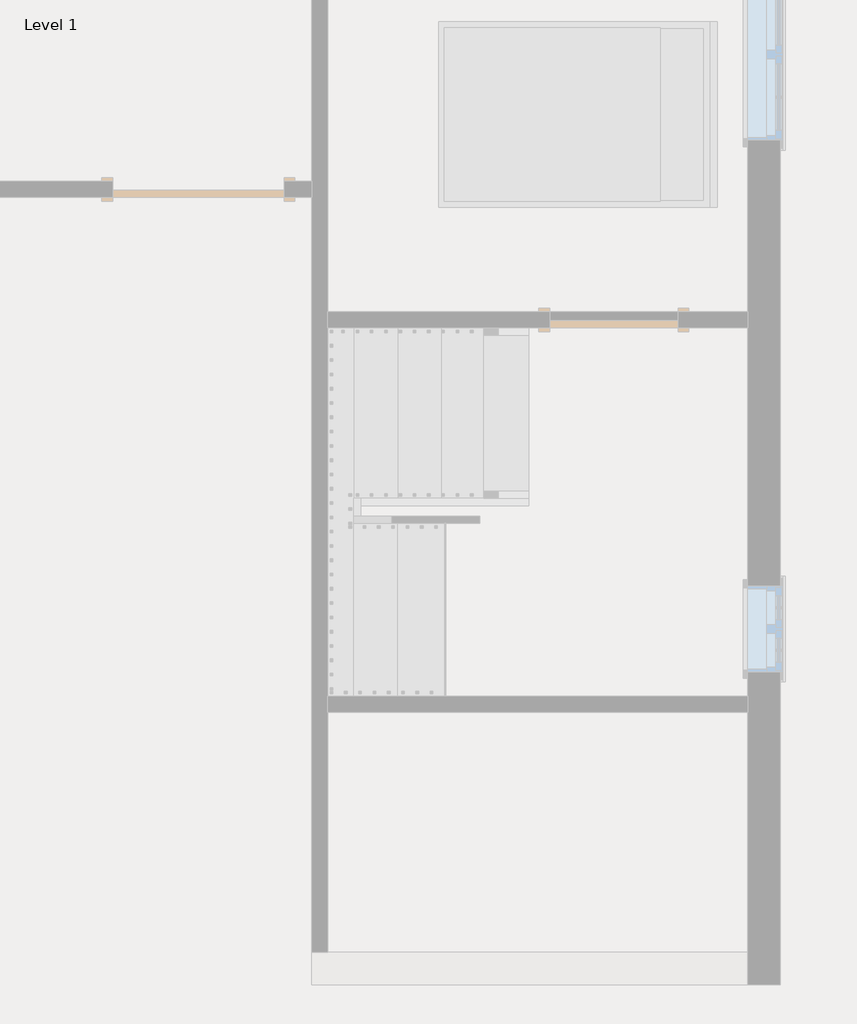
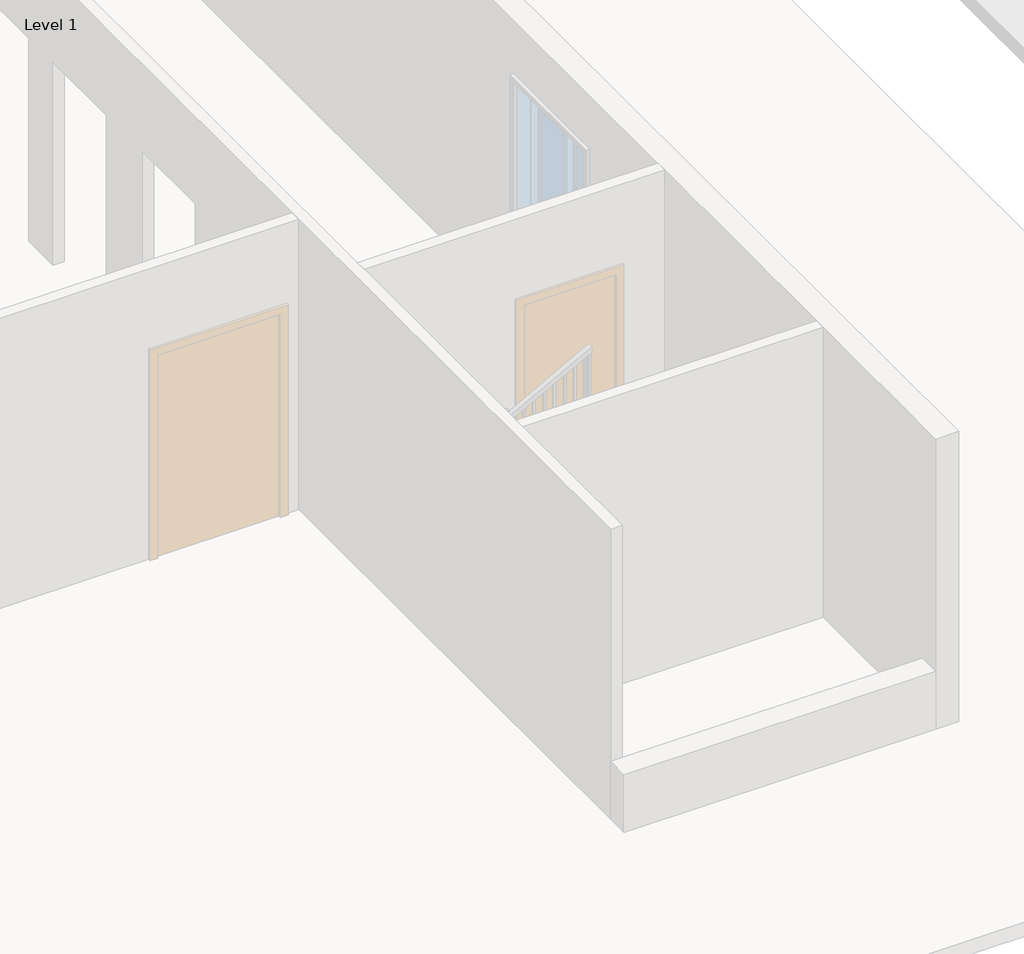
# One storey, part 4 of 7: 2 railings.
"""IFC4 building model written with IfcOpenShell, lengths in millimetres."""

from ifc_helpers import new_model, si_unit, frame, origin, place, context, project, spatial, polyline, outline, extrude, faceted_brep, element, save

model = new_model("IFC4")

# Units and contexts
model_context = context("Model", 3, world=origin())
ifc_project = project(units=[si_unit("LENGTHUNIT", "METRE", prefix="MILLI")], contexts=[model_context])

# Site, building, storey
site = spatial("IfcSite", under=ifc_project)
building = spatial("IfcBuilding", under=site)
storey = spatial("IfcBuildingStorey", under=building, Name="Level 1", Elevation=0.0)

# Railings
placement = place(None, origin())
element("IfcRailing", 1, ObjectType="Handrail - Rectangular", at=placement, inside=storey, context=model_context, shape_type="SolidModel", body=[
    faceted_brep([(7105.1820958, 5435.6, 1083.7333333), (7105.1820958, 5435.6, 1025.8977421), (7105.1820958, 5486.4, 1025.8977421), (7105.1820958, 5486.4, 1083.7333333), (5860.5820958, 5435.6, 1761.0666667), (5847.654197, 5435.6, 1710.2666667), (5847.654197, 5486.4, 1710.2666667), (5860.5820958, 5486.4, 1761.0666667), (5727.7, 5435.6, 1761.0666667), (5727.7, 5435.6, 1710.2666667), (5676.9, 5486.4, 1710.2666667), (5676.9, 5486.4, 1761.0666667), (5727.7, 2997.2, 1761.0666667), (5727.7, 2946.4, 1710.2666667), (5676.9, 2946.4, 1710.2666667), (5676.9, 2997.2, 1761.0666667), (5727.7, 2997.2, 1899.5526009), (5727.7, 2946.4, 1848.7526009), (5676.9, 2946.4, 1848.7526009), (5676.9, 2997.2, 1899.5526009), (5727.7, 2921.0, 1899.5526009), (5727.7, 2921.0, 1848.7526009), (5676.9, 2870.2, 1848.7526009), (5676.9, 2870.2, 1899.5526009), (5803.9, 2921.0, 1899.5526009), (5816.8278988, 2921.0, 1848.7526009), (5816.8278988, 2870.2, 1848.7526009), (5803.9, 2870.2, 1899.5526009), (7105.1820958, 2921.0, 2607.7333333), (7105.1820958, 2870.2, 2607.7333333), (7105.1820958, 2870.2, 2549.8977421), (7105.1820958, 2921.0, 2549.8977421)], [[[0, 1, 2, 3]], [[1, 0, 4, 5]], [[2, 1, 5, 6]], [[3, 2, 6, 7]], [[0, 3, 7, 4]], [[5, 4, 8, 9]], [[6, 5, 9, 10]], [[7, 6, 10, 11]], [[4, 7, 11, 8]], [[9, 8, 12, 13]], [[10, 9, 13, 14]], [[11, 10, 14, 15]], [[8, 11, 15, 12]], [[13, 12, 16, 17]], [[14, 13, 17, 18]], [[15, 14, 18, 19]], [[12, 15, 19, 16]], [[17, 16, 20, 21]], [[18, 17, 21, 22]], [[19, 18, 22, 23]], [[16, 19, 23, 20]], [[21, 20, 24, 25]], [[22, 21, 25, 26]], [[23, 22, 26, 27]], [[20, 23, 27, 24]], [[28, 29, 30, 31]], [[25, 24, 28, 31]], [[26, 25, 31, 30]], [[27, 26, 30, 29]], [[24, 27, 29, 28]]]),
    extrude(outline(polyline([(2510.4108873, 7032.625), (2500.0435403, 7013.575), (1524.0, 7013.575), (1524.0, 7032.625), (2510.4108873, 7032.625)])), frame((0.0, 2886.075, 0.0), z_axis=(0.0, 1.0, 0.0), x_axis=(0.0, 0.0, 1.0)), (0.0, 0.0, 1.0), 19.05),
    extrude(outline(polyline([(2455.1183703, 6931.025), (2444.7510233, 6911.975), (1524.0, 6911.975), (1524.0, 6931.025), (2455.1183703, 6931.025)])), frame((0.0, 2886.075, 0.0), z_axis=(0.0, 1.0, 0.0), x_axis=(0.0, 0.0, 1.0)), (0.0, 0.0, 1.0), 19.05),
    extrude(outline(polyline([(2399.8258533, 6829.425), (2389.4585063, 6810.375), (1524.0, 6810.375), (1524.0, 6829.425), (2399.8258533, 6829.425)])), frame((0.0, 2886.075, 0.0), z_axis=(0.0, 1.0, 0.0), x_axis=(0.0, 0.0, 1.0)), (0.0, 0.0, 1.0), 19.05),
    extrude(outline(polyline([(2344.5333363, 6727.825), (2334.1659893, 6708.775), (1354.6666667, 6708.775), (1354.6666667, 6727.825), (2344.5333363, 6727.825)])), frame((0.0, 2886.075, 0.0), z_axis=(0.0, 1.0, 0.0), x_axis=(0.0, 0.0, 1.0)), (0.0, 0.0, 1.0), 19.05),
    extrude(outline(polyline([(2289.2408192, 6626.225), (2278.8734723, 6607.175), (1354.6666667, 6607.175), (1354.6666667, 6626.225), (2289.2408192, 6626.225)])), frame((0.0, 2886.075, 0.0), z_axis=(0.0, 1.0, 0.0), x_axis=(0.0, 0.0, 1.0)), (0.0, 0.0, 1.0), 19.05),
    extrude(outline(polyline([(2233.9483022, 6524.625), (2223.5809553, 6505.575), (1354.6666667, 6505.575), (1354.6666667, 6524.625), (2233.9483022, 6524.625)])), frame((0.0, 2886.075, 0.0), z_axis=(0.0, 1.0, 0.0), x_axis=(0.0, 0.0, 1.0)), (0.0, 0.0, 1.0), 19.05),
    extrude(outline(polyline([(2178.6557852, 6423.025), (2168.2884383, 6403.975), (1185.3333333, 6403.975), (1185.3333333, 6423.025), (2178.6557852, 6423.025)])), frame((0.0, 2886.075, 0.0), z_axis=(0.0, 1.0, 0.0), x_axis=(0.0, 0.0, 1.0)), (0.0, 0.0, 1.0), 19.05),
    extrude(outline(polyline([(2123.3632682, 6321.425), (2112.9959213, 6302.375), (1185.3333333, 6302.375), (1185.3333333, 6321.425), (2123.3632682, 6321.425)])), frame((0.0, 2886.075, 0.0), z_axis=(0.0, 1.0, 0.0), x_axis=(0.0, 0.0, 1.0)), (0.0, 0.0, 1.0), 19.05),
    extrude(outline(polyline([(2068.0707512, 6219.825), (2057.7034043, 6200.775), (1185.3333333, 6200.775), (1185.3333333, 6219.825), (2068.0707512, 6219.825)])), frame((0.0, 2886.075, 0.0), z_axis=(0.0, 1.0, 0.0), x_axis=(0.0, 0.0, 1.0)), (0.0, 0.0, 1.0), 19.05),
    extrude(outline(polyline([(2012.7782342, 6118.225), (2002.4108873, 6099.175), (1016.0, 6099.175), (1016.0, 6118.225), (2012.7782342, 6118.225)])), frame((0.0, 2886.075, 0.0), z_axis=(0.0, 1.0, 0.0), x_axis=(0.0, 0.0, 1.0)), (0.0, 0.0, 1.0), 19.05),
    extrude(outline(polyline([(1957.4857172, 6016.625), (1947.1183703, 5997.575), (1016.0, 5997.575), (1016.0, 6016.625), (1957.4857172, 6016.625)])), frame((0.0, 2886.075, 0.0), z_axis=(0.0, 1.0, 0.0), x_axis=(0.0, 0.0, 1.0)), (0.0, 0.0, 1.0), 19.05),
    extrude(outline(polyline([(1902.1932002, 5915.025), (1891.8258533, 5895.975), (1016.0, 5895.975), (1016.0, 5915.025), (1902.1932002, 5915.025)])), frame((0.0, 2886.075, 0.0), z_axis=(0.0, 1.0, 0.0), x_axis=(0.0, 0.0, 1.0)), (0.0, 0.0, 1.0), 19.05),
    extrude(outline(polyline([(1846.9006832, 5813.425), (1836.5333363, 5794.375), (846.6666667, 5794.375), (846.6666667, 5813.425), (1846.9006832, 5813.425)])), frame((0.0, 2886.075, 0.0), z_axis=(0.0, 1.0, 0.0), x_axis=(0.0, 0.0, 1.0)), (0.0, 0.0, 1.0), 19.05),
    extrude(outline(polyline([(5692.775, 2930.525), (5711.825, 2930.525), (5711.825, 2911.475), (5692.775, 2911.475), (5692.775, 2930.525)])), frame((0.0, 0.0, 846.6666667), z_axis=(0.0, 0.0, 1.0), x_axis=(1.0, 0.0, 0.0)), (0.0, 0.0, 1.0), 1002.0859343),
    extrude(outline(polyline([(5692.775, 3032.125), (5711.825, 3032.125), (5711.825, 3013.075), (5692.775, 3013.075), (5692.775, 3032.125)])), frame((0.0, 0.0, 846.6666667), z_axis=(0.0, 0.0, 1.0), x_axis=(1.0, 0.0, 0.0)), (0.0, 0.0, 1.0), 863.6),
    extrude(outline(polyline([(5692.775, 3133.725), (5711.825, 3133.725), (5711.825, 3114.675), (5692.775, 3114.675), (5692.775, 3133.725)])), frame((0.0, 0.0, 846.6666667), z_axis=(0.0, 0.0, 1.0), x_axis=(1.0, 0.0, 0.0)), (0.0, 0.0, 1.0), 863.6),
    extrude(outline(polyline([(5692.775, 3235.325), (5711.825, 3235.325), (5711.825, 3216.275), (5692.775, 3216.275), (5692.775, 3235.325)])), frame((0.0, 0.0, 846.6666667), z_axis=(0.0, 0.0, 1.0), x_axis=(1.0, 0.0, 0.0)), (0.0, 0.0, 1.0), 863.6),
    extrude(outline(polyline([(5692.775, 3336.925), (5711.825, 3336.925), (5711.825, 3317.875), (5692.775, 3317.875), (5692.775, 3336.925)])), frame((0.0, 0.0, 846.6666667), z_axis=(0.0, 0.0, 1.0), x_axis=(1.0, 0.0, 0.0)), (0.0, 0.0, 1.0), 863.6),
    extrude(outline(polyline([(5692.775, 3438.525), (5711.825, 3438.525), (5711.825, 3419.475), (5692.775, 3419.475), (5692.775, 3438.525)])), frame((0.0, 0.0, 846.6666667), z_axis=(0.0, 0.0, 1.0), x_axis=(1.0, 0.0, 0.0)), (0.0, 0.0, 1.0), 863.6),
    extrude(outline(polyline([(5692.775, 3540.125), (5711.825, 3540.125), (5711.825, 3521.075), (5692.775, 3521.075), (5692.775, 3540.125)])), frame((0.0, 0.0, 846.6666667), z_axis=(0.0, 0.0, 1.0), x_axis=(1.0, 0.0, 0.0)), (0.0, 0.0, 1.0), 863.6),
    extrude(outline(polyline([(5692.775, 3641.725), (5711.825, 3641.725), (5711.825, 3622.675), (5692.775, 3622.675), (5692.775, 3641.725)])), frame((0.0, 0.0, 846.6666667), z_axis=(0.0, 0.0, 1.0), x_axis=(1.0, 0.0, 0.0)), (0.0, 0.0, 1.0), 863.6),
    extrude(outline(polyline([(5692.775, 3743.325), (5711.825, 3743.325), (5711.825, 3724.275), (5692.775, 3724.275), (5692.775, 3743.325)])), frame((0.0, 0.0, 846.6666667), z_axis=(0.0, 0.0, 1.0), x_axis=(1.0, 0.0, 0.0)), (0.0, 0.0, 1.0), 863.6),
    extrude(outline(polyline([(5692.775, 3844.925), (5711.825, 3844.925), (5711.825, 3825.875), (5692.775, 3825.875), (5692.775, 3844.925)])), frame((0.0, 0.0, 846.6666667), z_axis=(0.0, 0.0, 1.0), x_axis=(1.0, 0.0, 0.0)), (0.0, 0.0, 1.0), 863.6),
    extrude(outline(polyline([(5692.775, 3946.525), (5711.825, 3946.525), (5711.825, 3927.475), (5692.775, 3927.475), (5692.775, 3946.525)])), frame((0.0, 0.0, 846.6666667), z_axis=(0.0, 0.0, 1.0), x_axis=(1.0, 0.0, 0.0)), (0.0, 0.0, 1.0), 863.6),
    extrude(outline(polyline([(5692.775, 4048.125), (5711.825, 4048.125), (5711.825, 4029.075), (5692.775, 4029.075), (5692.775, 4048.125)])), frame((0.0, 0.0, 846.6666667), z_axis=(0.0, 0.0, 1.0), x_axis=(1.0, 0.0, 0.0)), (0.0, 0.0, 1.0), 863.6),
    extrude(outline(polyline([(5692.775, 4149.725), (5711.825, 4149.725), (5711.825, 4130.675), (5692.775, 4130.675), (5692.775, 4149.725)])), frame((0.0, 0.0, 846.6666667), z_axis=(0.0, 0.0, 1.0), x_axis=(1.0, 0.0, 0.0)), (0.0, 0.0, 1.0), 863.6),
    extrude(outline(polyline([(5692.775, 4251.325), (5711.825, 4251.325), (5711.825, 4232.275), (5692.775, 4232.275), (5692.775, 4251.325)])), frame((0.0, 0.0, 846.6666667), z_axis=(0.0, 0.0, 1.0), x_axis=(1.0, 0.0, 0.0)), (0.0, 0.0, 1.0), 863.6),
    extrude(outline(polyline([(5692.775, 4352.925), (5711.825, 4352.925), (5711.825, 4333.875), (5692.775, 4333.875), (5692.775, 4352.925)])), frame((0.0, 0.0, 846.6666667), z_axis=(0.0, 0.0, 1.0), x_axis=(1.0, 0.0, 0.0)), (0.0, 0.0, 1.0), 863.6),
    extrude(outline(polyline([(5692.775, 4454.525), (5711.825, 4454.525), (5711.825, 4435.475), (5692.775, 4435.475), (5692.775, 4454.525)])), frame((0.0, 0.0, 846.6666667), z_axis=(0.0, 0.0, 1.0), x_axis=(1.0, 0.0, 0.0)), (0.0, 0.0, 1.0), 863.6),
    extrude(outline(polyline([(5692.775, 4556.125), (5711.825, 4556.125), (5711.825, 4537.075), (5692.775, 4537.075), (5692.775, 4556.125)])), frame((0.0, 0.0, 846.6666667), z_axis=(0.0, 0.0, 1.0), x_axis=(1.0, 0.0, 0.0)), (0.0, 0.0, 1.0), 863.6),
    extrude(outline(polyline([(5692.775, 4657.725), (5711.825, 4657.725), (5711.825, 4638.675), (5692.775, 4638.675), (5692.775, 4657.725)])), frame((0.0, 0.0, 846.6666667), z_axis=(0.0, 0.0, 1.0), x_axis=(1.0, 0.0, 0.0)), (0.0, 0.0, 1.0), 863.6),
    extrude(outline(polyline([(5692.775, 4759.325), (5711.825, 4759.325), (5711.825, 4740.275), (5692.775, 4740.275), (5692.775, 4759.325)])), frame((0.0, 0.0, 846.6666667), z_axis=(0.0, 0.0, 1.0), x_axis=(1.0, 0.0, 0.0)), (0.0, 0.0, 1.0), 863.6),
    extrude(outline(polyline([(5692.775, 4860.925), (5711.825, 4860.925), (5711.825, 4841.875), (5692.775, 4841.875), (5692.775, 4860.925)])), frame((0.0, 0.0, 846.6666667), z_axis=(0.0, 0.0, 1.0), x_axis=(1.0, 0.0, 0.0)), (0.0, 0.0, 1.0), 863.6),
    extrude(outline(polyline([(5692.775, 4962.525), (5711.825, 4962.525), (5711.825, 4943.475), (5692.775, 4943.475), (5692.775, 4962.525)])), frame((0.0, 0.0, 846.6666667), z_axis=(0.0, 0.0, 1.0), x_axis=(1.0, 0.0, 0.0)), (0.0, 0.0, 1.0), 863.6),
    extrude(outline(polyline([(5692.775, 5064.125), (5711.825, 5064.125), (5711.825, 5045.075), (5692.775, 5045.075), (5692.775, 5064.125)])), frame((0.0, 0.0, 846.6666667), z_axis=(0.0, 0.0, 1.0), x_axis=(1.0, 0.0, 0.0)), (0.0, 0.0, 1.0), 863.6),
    extrude(outline(polyline([(5692.775, 5165.725), (5711.825, 5165.725), (5711.825, 5146.675), (5692.775, 5146.675), (5692.775, 5165.725)])), frame((0.0, 0.0, 846.6666667), z_axis=(0.0, 0.0, 1.0), x_axis=(1.0, 0.0, 0.0)), (0.0, 0.0, 1.0), 863.6),
    extrude(outline(polyline([(5692.775, 5267.325), (5711.825, 5267.325), (5711.825, 5248.275), (5692.775, 5248.275), (5692.775, 5267.325)])), frame((0.0, 0.0, 846.6666667), z_axis=(0.0, 0.0, 1.0), x_axis=(1.0, 0.0, 0.0)), (0.0, 0.0, 1.0), 863.6),
    extrude(outline(polyline([(5692.775, 5368.925), (5711.825, 5368.925), (5711.825, 5349.875), (5692.775, 5349.875), (5692.775, 5368.925)])), frame((0.0, 0.0, 846.6666667), z_axis=(0.0, 0.0, 1.0), x_axis=(1.0, 0.0, 0.0)), (0.0, 0.0, 1.0), 863.6),
    extrude(outline(polyline([(5793.9070958, 5470.525), (5793.9070958, 5451.475), (5774.8570958, 5451.475), (5774.8570958, 5470.525), (5793.9070958, 5470.525)])), frame((0.0, 0.0, 846.6666667), z_axis=(0.0, 0.0, 1.0), x_axis=(1.0, 0.0, 0.0)), (0.0, 0.0, 1.0), 863.6),
    extrude(outline(polyline([(1684.2242727, 5895.5070958), (1694.5916197, 5876.4570958), (677.3333333, 5876.4570958), (677.3333333, 5895.5070958), (1684.2242727, 5895.5070958)])), frame((0.0, 5451.475, 0.0), z_axis=(0.0, 1.0, 0.0), x_axis=(0.0, 0.0, 1.0)), (0.0, 0.0, 1.0), 19.05),
    extrude(outline(polyline([(1628.9317557, 5997.1070958), (1639.2991027, 5978.0570958), (677.3333333, 5978.0570958), (677.3333333, 5997.1070958), (1628.9317557, 5997.1070958)])), frame((0.0, 5451.475, 0.0), z_axis=(0.0, 1.0, 0.0), x_axis=(0.0, 0.0, 1.0)), (0.0, 0.0, 1.0), 19.05),
    extrude(outline(polyline([(1573.6392387, 6098.7070958), (1584.0065857, 6079.6570958), (677.3333333, 6079.6570958), (677.3333333, 6098.7070958), (1573.6392387, 6098.7070958)])), frame((0.0, 5451.475, 0.0), z_axis=(0.0, 1.0, 0.0), x_axis=(0.0, 0.0, 1.0)), (0.0, 0.0, 1.0), 19.05),
    extrude(outline(polyline([(1518.3467217, 6200.3070958), (1528.7140687, 6181.2570958), (508.0, 6181.2570958), (508.0, 6200.3070958), (1518.3467217, 6200.3070958)])), frame((0.0, 5451.475, 0.0), z_axis=(0.0, 1.0, 0.0), x_axis=(0.0, 0.0, 1.0)), (0.0, 0.0, 1.0), 19.05),
    extrude(outline(polyline([(1463.0542047, 6301.9070958), (1473.4215517, 6282.8570958), (508.0, 6282.8570958), (508.0, 6301.9070958), (1463.0542047, 6301.9070958)])), frame((0.0, 5451.475, 0.0), z_axis=(0.0, 1.0, 0.0), x_axis=(0.0, 0.0, 1.0)), (0.0, 0.0, 1.0), 19.05),
    extrude(outline(polyline([(1407.7616877, 6403.5070958), (1418.1290347, 6384.4570958), (508.0, 6384.4570958), (508.0, 6403.5070958), (1407.7616877, 6403.5070958)])), frame((0.0, 5451.475, 0.0), z_axis=(0.0, 1.0, 0.0), x_axis=(0.0, 0.0, 1.0)), (0.0, 0.0, 1.0), 19.05),
    extrude(outline(polyline([(1352.4691707, 6505.1070958), (1362.8365176, 6486.0570958), (338.6666667, 6486.0570958), (338.6666667, 6505.1070958), (1352.4691707, 6505.1070958)])), frame((0.0, 5451.475, 0.0), z_axis=(0.0, 1.0, 0.0), x_axis=(0.0, 0.0, 1.0)), (0.0, 0.0, 1.0), 19.05),
    extrude(outline(polyline([(1297.1766537, 6606.7070958), (1307.5440006, 6587.6570958), (338.6666667, 6587.6570958), (338.6666667, 6606.7070958), (1297.1766537, 6606.7070958)])), frame((0.0, 5451.475, 0.0), z_axis=(0.0, 1.0, 0.0), x_axis=(0.0, 0.0, 1.0)), (0.0, 0.0, 1.0), 19.05),
    extrude(outline(polyline([(1241.8841367, 6708.3070958), (1252.2514836, 6689.2570958), (338.6666667, 6689.2570958), (338.6666667, 6708.3070958), (1241.8841367, 6708.3070958)])), frame((0.0, 5451.475, 0.0), z_axis=(0.0, 1.0, 0.0), x_axis=(0.0, 0.0, 1.0)), (0.0, 0.0, 1.0), 19.05),
    extrude(outline(polyline([(1186.5916197, 6809.9070958), (1196.9589666, 6790.8570958), (169.3333333, 6790.8570958), (169.3333333, 6809.9070958), (1186.5916197, 6809.9070958)])), frame((0.0, 5451.475, 0.0), z_axis=(0.0, 1.0, 0.0), x_axis=(0.0, 0.0, 1.0)), (0.0, 0.0, 1.0), 19.05),
    extrude(outline(polyline([(1131.2991027, 6911.5070958), (1141.6664496, 6892.4570958), (169.3333333, 6892.4570958), (169.3333333, 6911.5070958), (1131.2991027, 6911.5070958)])), frame((0.0, 5451.475, 0.0), z_axis=(0.0, 1.0, 0.0), x_axis=(0.0, 0.0, 1.0)), (0.0, 0.0, 1.0), 19.05),
    extrude(outline(polyline([(1076.0065857, 7013.1070958), (1086.3739326, 6994.0570958), (169.3333333, 6994.0570958), (169.3333333, 7013.1070958), (1076.0065857, 7013.1070958)])), frame((0.0, 5451.475, 0.0), z_axis=(0.0, 1.0, 0.0), x_axis=(0.0, 0.0, 1.0)), (0.0, 0.0, 1.0), 19.05),
    extrude(outline(polyline([(5692.775, 2905.125), (5711.825, 2905.125), (5711.825, 2886.075), (5692.775, 2886.075), (5692.775, 2905.125)])), frame((0.0, 0.0, 846.6666667), z_axis=(0.0, 0.0, 1.0), x_axis=(1.0, 0.0, 0.0)), (0.0, 0.0, 1.0), 1002.0859343),
    extrude(outline(polyline([(5711.825, 5470.525), (5711.825, 5451.475), (5692.775, 5451.475), (5692.775, 5470.525), (5711.825, 5470.525)])), frame((0.0, 0.0, 846.6666667), z_axis=(0.0, 0.0, 1.0), x_axis=(1.0, 0.0, 0.0)), (0.0, 0.0, 1.0), 863.6),
    extrude(outline(polyline([(2549.8977421, 7105.1820958), (2539.5303952, 7086.1320958), (1524.0, 7086.1320958), (1524.0, 7105.1820958), (2549.8977421, 7105.1820958)])), frame((0.0, 2886.075, 0.0), z_axis=(0.0, 1.0, 0.0), x_axis=(0.0, 0.0, 1.0)), (0.0, 0.0, 1.0), 19.05),
    extrude(outline(polyline([(1025.8977421, 7105.1820958), (1036.2650891, 7086.1320958), (169.3333333, 7086.1320958), (169.3333333, 7105.1820958), (1025.8977421, 7105.1820958)])), frame((0.0, 5451.475, 0.0), z_axis=(0.0, 1.0, 0.0), x_axis=(0.0, 0.0, 1.0)), (0.0, 0.0, 1.0), 19.05),
])
element("IfcRailing", 2, ObjectType="Handrail - Rectangular", at=placement, inside=storey, context=model_context, shape_type="SolidModel", body=[
    faceted_brep([(7105.1820958, 4274.6882626, 1083.7333333), (7105.1820958, 4274.6882626, 1025.8977421), (7105.1820958, 4325.4882626, 1025.8977421), (7105.1820958, 4325.4882626, 1083.7333333), (5936.7820958, 4274.6882626, 1719.5972789), (5885.9820958, 4274.6882626, 1689.4079462), (5885.9820958, 4325.4882626, 1689.4079462), (5936.7820958, 4325.4882626, 1719.5972789), (5936.7820958, 4274.6882626, 1761.0666667), (5885.9820958, 4274.6882626, 1710.2666667), (5885.9820958, 4325.4882626, 1710.2666667), (5936.7820958, 4325.4882626, 1761.0666667), (5860.5820958, 4274.6882626, 1761.0666667), (5860.5820958, 4274.6882626, 1710.2666667), (5809.7820958, 4325.4882626, 1710.2666667), (5809.7820958, 4325.4882626, 1761.0666667), (5860.5820958, 4198.4882626, 1761.0666667), (5860.5820958, 4198.4882626, 1710.2666667), (5809.7820958, 4198.4882626, 1710.2666667), (5809.7820958, 4198.4882626, 1761.0666667), (5860.5820958, 4173.0882626, 1761.0666667), (5860.5820958, 4122.2882626, 1710.2666667), (5809.7820958, 4122.2882626, 1710.2666667), (5809.7820958, 4173.0882626, 1761.0666667), (5860.5820958, 4173.0882626, 1971.8693878), (5860.5820958, 4122.2882626, 1921.0693878), (5809.7820958, 4122.2882626, 1921.0693878), (5809.7820958, 4173.0882626, 1971.8693878), (5860.5820958, 4096.8882626, 1971.8693878), (5860.5820958, 4096.8882626, 1921.0693878), (5809.7820958, 4046.0882626, 1921.0693878), (5809.7820958, 4046.0882626, 1971.8693878), (5936.7820958, 4096.8882626, 1971.8693878), (5949.7099946, 4096.8882626, 1921.0693878), (5949.7099946, 4046.0882626, 1921.0693878), (5936.7820958, 4046.0882626, 1971.8693878), (7105.1820958, 4096.8882626, 2607.7333333), (7105.1820958, 4046.0882626, 2607.7333333), (7105.1820958, 4046.0882626, 2549.8977421), (7105.1820958, 4096.8882626, 2549.8977421)], [[[0, 1, 2, 3]], [[1, 0, 4, 5]], [[2, 1, 5, 6]], [[3, 2, 6, 7]], [[0, 3, 7, 4]], [[5, 4, 8, 9]], [[6, 5, 9, 10]], [[7, 6, 10, 11]], [[4, 7, 11, 8]], [[9, 8, 12, 13]], [[10, 9, 13, 14]], [[11, 10, 14, 15]], [[8, 11, 15, 12]], [[13, 12, 16, 17]], [[14, 13, 17, 18]], [[15, 14, 18, 19]], [[12, 15, 19, 16]], [[17, 16, 20, 21]], [[18, 17, 21, 22]], [[19, 18, 22, 23]], [[16, 19, 23, 20]], [[21, 20, 24, 25]], [[22, 21, 25, 26]], [[23, 22, 26, 27]], [[20, 23, 27, 24]], [[25, 24, 28, 29]], [[26, 25, 29, 30]], [[27, 26, 30, 31]], [[24, 27, 31, 28]], [[29, 28, 32, 33]], [[30, 29, 33, 34]], [[31, 30, 34, 35]], [[28, 31, 35, 32]], [[36, 37, 38, 39]], [[33, 32, 36, 39]], [[34, 33, 39, 38]], [[35, 34, 38, 37]], [[32, 35, 37, 36]]]),
    extrude(outline(polyline([(2517.0678102, 7044.8570958), (1524.0, 7044.8570958), (1524.0, 7063.9070958), (2527.4351571, 7063.9070958), (2517.0678102, 7044.8570958)])), frame((0.0, 4061.9632626, 0.0), z_axis=(0.0, 1.0, 0.0), x_axis=(0.0, 0.0, 1.0)), (0.0, 0.0, 1.0), 19.05),
    extrude(outline(polyline([(2461.7752932, 6943.2570958), (1524.0, 6943.2570958), (1524.0, 6962.3070958), (2472.1426401, 6962.3070958), (2461.7752932, 6943.2570958)])), frame((0.0, 4061.9632626, 0.0), z_axis=(0.0, 1.0, 0.0), x_axis=(0.0, 0.0, 1.0)), (0.0, 0.0, 1.0), 19.05),
    extrude(outline(polyline([(2406.4827761, 6841.6570958), (1524.0, 6841.6570958), (1524.0, 6860.7070958), (2416.8501231, 6860.7070958), (2406.4827761, 6841.6570958)])), frame((0.0, 4061.9632626, 0.0), z_axis=(0.0, 1.0, 0.0), x_axis=(0.0, 0.0, 1.0)), (0.0, 0.0, 1.0), 19.05),
    extrude(outline(polyline([(2351.1902591, 6740.0570958), (1354.6666667, 6740.0570958), (1354.6666667, 6759.1070958), (2361.5576061, 6759.1070958), (2351.1902591, 6740.0570958)])), frame((0.0, 4061.9632626, 0.0), z_axis=(0.0, 1.0, 0.0), x_axis=(0.0, 0.0, 1.0)), (0.0, 0.0, 1.0), 19.05),
    extrude(outline(polyline([(2295.8977421, 6638.4570958), (1354.6666667, 6638.4570958), (1354.6666667, 6657.5070958), (2306.2650891, 6657.5070958), (2295.8977421, 6638.4570958)])), frame((0.0, 4061.9632626, 0.0), z_axis=(0.0, 1.0, 0.0), x_axis=(0.0, 0.0, 1.0)), (0.0, 0.0, 1.0), 19.05),
    extrude(outline(polyline([(2240.6052251, 6536.8570958), (1354.6666667, 6536.8570958), (1354.6666667, 6555.9070958), (2250.9725721, 6555.9070958), (2240.6052251, 6536.8570958)])), frame((0.0, 4061.9632626, 0.0), z_axis=(0.0, 1.0, 0.0), x_axis=(0.0, 0.0, 1.0)), (0.0, 0.0, 1.0), 19.05),
    extrude(outline(polyline([(2185.3127081, 6435.2570958), (1185.3333333, 6435.2570958), (1185.3333333, 6454.3070958), (2195.6800551, 6454.3070958), (2185.3127081, 6435.2570958)])), frame((0.0, 4061.9632626, 0.0), z_axis=(0.0, 1.0, 0.0), x_axis=(0.0, 0.0, 1.0)), (0.0, 0.0, 1.0), 19.05),
    extrude(outline(polyline([(2130.0201911, 6333.6570958), (1185.3333333, 6333.6570958), (1185.3333333, 6352.7070958), (2140.3875381, 6352.7070958), (2130.0201911, 6333.6570958)])), frame((0.0, 4061.9632626, 0.0), z_axis=(0.0, 1.0, 0.0), x_axis=(0.0, 0.0, 1.0)), (0.0, 0.0, 1.0), 19.05),
    extrude(outline(polyline([(2074.7276741, 6232.0570958), (1185.3333333, 6232.0570958), (1185.3333333, 6251.1070958), (2085.095021, 6251.1070958), (2074.7276741, 6232.0570958)])), frame((0.0, 4061.9632626, 0.0), z_axis=(0.0, 1.0, 0.0), x_axis=(0.0, 0.0, 1.0)), (0.0, 0.0, 1.0), 19.05),
    extrude(outline(polyline([(2019.4351571, 6130.4570958), (1016.0, 6130.4570958), (1016.0, 6149.5070958), (2029.802504, 6149.5070958), (2019.4351571, 6130.4570958)])), frame((0.0, 4061.9632626, 0.0), z_axis=(0.0, 1.0, 0.0), x_axis=(0.0, 0.0, 1.0)), (0.0, 0.0, 1.0), 19.05),
    extrude(outline(polyline([(1964.1426401, 6028.8570958), (1016.0, 6028.8570958), (1016.0, 6047.9070958), (1974.509987, 6047.9070958), (1964.1426401, 6028.8570958)])), frame((0.0, 4061.9632626, 0.0), z_axis=(0.0, 1.0, 0.0), x_axis=(0.0, 0.0, 1.0)), (0.0, 0.0, 1.0), 19.05),
    extrude(outline(polyline([(1908.8501231, 5927.2570958), (1016.0, 5927.2570958), (1016.0, 5946.3070958), (1919.21747, 5946.3070958), (1908.8501231, 5927.2570958)])), frame((0.0, 4061.9632626, 0.0), z_axis=(0.0, 1.0, 0.0), x_axis=(0.0, 0.0, 1.0)), (0.0, 0.0, 1.0), 19.05),
    extrude(outline(polyline([(5844.7070958, 4106.4132626), (5844.7070958, 4087.3632626), (5825.6570958, 4087.3632626), (5825.6570958, 4106.4132626), (5844.7070958, 4106.4132626)])), frame((0.0, 0.0, 846.6666667), z_axis=(0.0, 0.0, 1.0), x_axis=(1.0, 0.0, 0.0)), (0.0, 0.0, 1.0), 1074.4027211),
    extrude(outline(polyline([(5844.7070958, 4208.0132626), (5844.7070958, 4188.9632626), (5825.6570958, 4188.9632626), (5825.6570958, 4208.0132626), (5844.7070958, 4208.0132626)])), frame((0.0, 0.0, 846.6666667), z_axis=(0.0, 0.0, 1.0), x_axis=(1.0, 0.0, 0.0)), (0.0, 0.0, 1.0), 863.6),
    extrude(outline(polyline([(5895.5070958, 4290.5632626), (5876.4570958, 4290.5632626), (5876.4570958, 4309.6132626), (5895.5070958, 4309.6132626), (5895.5070958, 4290.5632626)])), frame((0.0, 0.0, 677.3333333), z_axis=(0.0, 0.0, 1.0), x_axis=(1.0, 0.0, 0.0)), (0.0, 0.0, 1.0), 1032.9333333),
    extrude(outline(polyline([(1639.2991027, 5978.0570958), (677.3333333, 5978.0570958), (677.3333333, 5997.1070958), (1628.9317557, 5997.1070958), (1639.2991027, 5978.0570958)])), frame((0.0, 4290.5632626, 0.0), z_axis=(0.0, 1.0, 0.0), x_axis=(0.0, 0.0, 1.0)), (0.0, 0.0, 1.0), 19.05),
    extrude(outline(polyline([(1584.0065857, 6079.6570958), (677.3333333, 6079.6570958), (677.3333333, 6098.7070958), (1573.6392387, 6098.7070958), (1584.0065857, 6079.6570958)])), frame((0.0, 4290.5632626, 0.0), z_axis=(0.0, 1.0, 0.0), x_axis=(0.0, 0.0, 1.0)), (0.0, 0.0, 1.0), 19.05),
    extrude(outline(polyline([(1528.7140687, 6181.2570958), (508.0, 6181.2570958), (508.0, 6200.3070958), (1518.3467217, 6200.3070958), (1528.7140687, 6181.2570958)])), frame((0.0, 4290.5632626, 0.0), z_axis=(0.0, 1.0, 0.0), x_axis=(0.0, 0.0, 1.0)), (0.0, 0.0, 1.0), 19.05),
    extrude(outline(polyline([(1473.4215517, 6282.8570958), (508.0, 6282.8570958), (508.0, 6301.9070958), (1463.0542047, 6301.9070958), (1473.4215517, 6282.8570958)])), frame((0.0, 4290.5632626, 0.0), z_axis=(0.0, 1.0, 0.0), x_axis=(0.0, 0.0, 1.0)), (0.0, 0.0, 1.0), 19.05),
    extrude(outline(polyline([(1418.1290347, 6384.4570958), (508.0, 6384.4570958), (508.0, 6403.5070958), (1407.7616877, 6403.5070958), (1418.1290347, 6384.4570958)])), frame((0.0, 4290.5632626, 0.0), z_axis=(0.0, 1.0, 0.0), x_axis=(0.0, 0.0, 1.0)), (0.0, 0.0, 1.0), 19.05),
    extrude(outline(polyline([(1362.8365176, 6486.0570958), (338.6666667, 6486.0570958), (338.6666667, 6505.1070958), (1352.4691707, 6505.1070958), (1362.8365176, 6486.0570958)])), frame((0.0, 4290.5632626, 0.0), z_axis=(0.0, 1.0, 0.0), x_axis=(0.0, 0.0, 1.0)), (0.0, 0.0, 1.0), 19.05),
    extrude(outline(polyline([(1307.5440006, 6587.6570958), (338.6666667, 6587.6570958), (338.6666667, 6606.7070958), (1297.1766537, 6606.7070958), (1307.5440006, 6587.6570958)])), frame((0.0, 4290.5632626, 0.0), z_axis=(0.0, 1.0, 0.0), x_axis=(0.0, 0.0, 1.0)), (0.0, 0.0, 1.0), 19.05),
    extrude(outline(polyline([(1252.2514836, 6689.2570958), (338.6666667, 6689.2570958), (338.6666667, 6708.3070958), (1241.8841367, 6708.3070958), (1252.2514836, 6689.2570958)])), frame((0.0, 4290.5632626, 0.0), z_axis=(0.0, 1.0, 0.0), x_axis=(0.0, 0.0, 1.0)), (0.0, 0.0, 1.0), 19.05),
    extrude(outline(polyline([(1196.9589666, 6790.8570958), (169.3333333, 6790.8570958), (169.3333333, 6809.9070958), (1186.5916197, 6809.9070958), (1196.9589666, 6790.8570958)])), frame((0.0, 4290.5632626, 0.0), z_axis=(0.0, 1.0, 0.0), x_axis=(0.0, 0.0, 1.0)), (0.0, 0.0, 1.0), 19.05),
    extrude(outline(polyline([(1141.6664496, 6892.4570958), (169.3333333, 6892.4570958), (169.3333333, 6911.5070958), (1131.2991027, 6911.5070958), (1141.6664496, 6892.4570958)])), frame((0.0, 4290.5632626, 0.0), z_axis=(0.0, 1.0, 0.0), x_axis=(0.0, 0.0, 1.0)), (0.0, 0.0, 1.0), 19.05),
    extrude(outline(polyline([(1086.3739326, 6994.0570958), (169.3333333, 6994.0570958), (169.3333333, 7013.1070958), (1076.0065857, 7013.1070958), (1086.3739326, 6994.0570958)])), frame((0.0, 4290.5632626, 0.0), z_axis=(0.0, 1.0, 0.0), x_axis=(0.0, 0.0, 1.0)), (0.0, 0.0, 1.0), 19.05),
    extrude(outline(polyline([(5844.7070958, 4081.0132626), (5844.7070958, 4061.9632626), (5825.6570958, 4061.9632626), (5825.6570958, 4081.0132626), (5844.7070958, 4081.0132626)])), frame((0.0, 0.0, 846.6666667), z_axis=(0.0, 0.0, 1.0), x_axis=(1.0, 0.0, 0.0)), (0.0, 0.0, 1.0), 1074.4027211),
    extrude(outline(polyline([(5844.7070958, 4290.5632626), (5825.6570958, 4290.5632626), (5825.6570958, 4309.6132626), (5844.7070958, 4309.6132626), (5844.7070958, 4290.5632626)])), frame((0.0, 0.0, 846.6666667), z_axis=(0.0, 0.0, 1.0), x_axis=(1.0, 0.0, 0.0)), (0.0, 0.0, 1.0), 863.6),
    extrude(outline(polyline([(2539.5303952, 7086.1320958), (1524.0, 7086.1320958), (1524.0, 7105.1820958), (2549.8977421, 7105.1820958), (2539.5303952, 7086.1320958)])), frame((0.0, 4061.9632626, 0.0), z_axis=(0.0, 1.0, 0.0), x_axis=(0.0, 0.0, 1.0)), (0.0, 0.0, 1.0), 19.05),
    extrude(outline(polyline([(1036.2650891, 7086.1320958), (169.3333333, 7086.1320958), (169.3333333, 7105.1820958), (1025.8977421, 7105.1820958), (1036.2650891, 7086.1320958)])), frame((0.0, 4290.5632626, 0.0), z_axis=(0.0, 1.0, 0.0), x_axis=(0.0, 0.0, 1.0)), (0.0, 0.0, 1.0), 19.05),
])

save(model, "model.ifc")

# Revit data of these elements
# Type "Handrail - Rectangular"
#   Assembly Code = "C2010400"
#   built-in parameter 1008612 = 0.0416667 (stored number, unit not read)
#   built-in parameter 1008611 = 0.0416667 (stored number, unit not read)
#   built-in parameter 1008609 = 0.333333 (stored number, unit not read)
#   built-in parameter 1008604 = 0.166667 (stored number, unit not read)
#   built-in parameter 1008603 = 0.166667 (stored number, unit not read)
#   Railing Height = 3' - 0"
#   built-in parameter 1008630 = 2
#   built-in parameter 1008610 = 2
#   built-in parameter 1008618 = Baluster - Square : 3/4"
# Elements 1, 2 (IfcRailing, "Handrail - Rectangular")
#   Phase Created = New Construction
